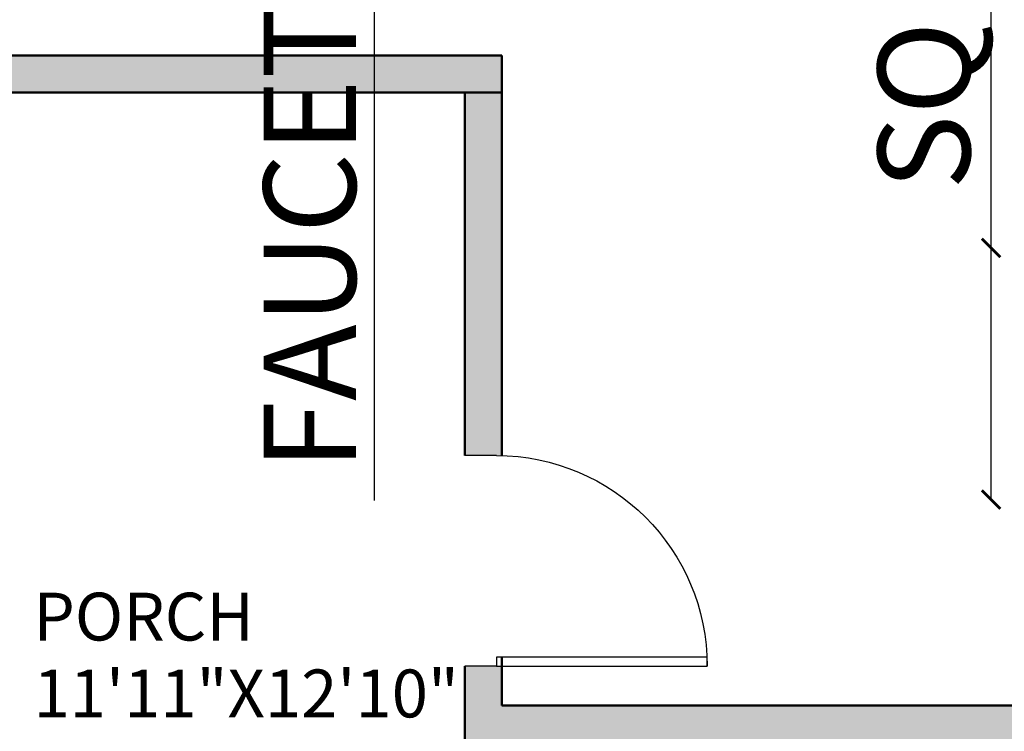
# Model space of a CAD drawing. Units: inches. Extents: x 2419 to 2878, y 1068 to 1713.
# Tile 9 of 20: x 2574 to 2708, y 1207 to 1304. Entities that reach past the tile are written whole.
import ezdxf

# ---------------------------------------------------------------- set-up
doc = ezdxf.new("R2010")
doc.units = ezdxf.units.IN
for name, color, linetype, lineweight in [('A-ANNO-DIMS', 2, 'Continuous', 18), ('A-AREA-IDEN', 7, 'Continuous', 18), ('A-DOOR', 4, 'Continuous', 25), ('A-FLOR-PRKG-PATT', 1, 'Continuous', 13), ('A-FURN-PATT', 254, 'Continuous', 13), ('A-WALL', 7, 'Continuous', 50)]:
    doc.layers.add(name, color=color, linetype=linetype, lineweight=lineweight)
doc.layers.add('A-FLOR-FIXT-PATT', color=254, linetype='Continuous', lineweight=13, true_color=0xd7ebd2)
doc.layers.add('A-WALL-PATT', color=18, linetype='Continuous', lineweight=13, true_color=0x000000)
doc.styles.get("Standard").update_dxf_attribs({"font": 'arial.ttf'})
doc.dimstyles.new('ISO-25', dxfattribs={"dimtxt": 12.5, "dimasz": 2.5, "dimexe": 1.25, "dimexo": 0.625, "dimtad": 1, "dimdec": 0, "dimlunit": 4, "dimtxsty": 'Standard', "dimblk": 'ARCHTICK', "dimcen": 2.5, "dimse1": 1, "dimse2": 1, "dimclrd": 4, "dimadec": 0, "dimazin": 0, "dimtfac": 1, "dimtdec": 0, "dimtmove": 0, "dimatfit": 3, "dimfxl": 1, "dimarcsym": 0})

# ---------------------------------------------------------------- blocks, each defined once
blk = doc.blocks.new('*U3')
for p, q in [((0, 0), (0, -6)), ((40, 0), (40, -6))]:
    blk.add_line(p, q)
blk.add_lwpolyline([(0, 0), (0, 40), (1.75, 40), (1.75, 0)], close=True)
blk.add_arc((0, 0), 40, 0, 90)
blk = doc.blocks.new('_ArchTick')
at = {"color": 0, "linetype": 'ByBlock', "const_width": 0.15}
blk.add_lwpolyline([(-0.5, -0.5), (0.5, 0.5)], dxfattribs=at)
blk = doc.blocks.new('*D20')
at = {"layer": 'A-ANNO-DIMS', "color": 4, "lineweight": -2, "transparency": 16777216}
for p, q in [((2622.22, 1404.52), (2622.22, 1392.52)), ((2622.22, 1392.52), (2622.22, 1238.58))]:
    blk.add_line(p, q, dxfattribs=at)
at = {"layer": 'Defpoints', "color": 0, "transparency": 16777216}
for p in [(2624.02, 1404.52), (2622.22, 1392.52), (2624.02, 1392.52)]:
    blk.add_point(p, dxfattribs=at)
at = {"layer": 'A-ANNO-DIMS', "color": 4, "lineweight": -2, "transparency": 16777216, "xscale": 2.5, "yscale": 2.5, "zscale": 2.5}
for p, rotation in [((2622.22, 1404.52), 90), ((2622.22, 1392.52), 270)]:
    blk.add_blockref('_ArchTick', p, dxfattribs=dict(at, rotation=rotation))
at = {"layer": 'A-ANNO-DIMS', "color": 0, "transparency": 16777216, "insert": (2615.13, 1314.3), "char_height": 12.5, "attachment_point": 5, "rotation": 90}
blk.add_mtext('FAUCET 1\'-0" TYP.', dxfattribs=at)
blk = doc.blocks.new('*D32')
at = {"layer": 'A-ANNO-DIMS', "color": 4, "lineweight": -2, "transparency": 16777216}
for p, q in [((2705.74, 1272.77), (2705.74, 1458.17)), ((2705.74, 1238.68), (2705.74, 1272.77))]:
    blk.add_line(p, q, dxfattribs=at)
at = {"layer": 'Defpoints', "color": 0, "transparency": 16777216}
for p in [(2705.74, 1272.77), (2710.85, 1272.77), (2710.85, 1238.68)]:
    blk.add_point(p, dxfattribs=at)
at = {"layer": 'A-ANNO-DIMS', "color": 4, "lineweight": -2, "transparency": 16777216, "xscale": 2.5, "yscale": 2.5, "zscale": 2.5}
for p, rotation in [((2705.74, 1272.77), 90), ((2705.74, 1238.68), 270)]:
    blk.add_blockref('_ArchTick', p, dxfattribs=dict(at, rotation=rotation))
at = {"layer": 'A-ANNO-DIMS', "color": 0, "transparency": 16777216, "insert": (2698.27, 1366.72), "char_height": 12.5, "attachment_point": 5, "rotation": 90}
blk.add_mtext('SQUARE TABLE 2\'-10"', dxfattribs=at)
blk = doc.blocks.new('*D36')
at = {"layer": 'A-ANNO-DIMS', "color": 4, "lineweight": -2, "transparency": 16777216}
blk.add_line((2656.74, 1605.01), (2736.32, 1605.01), dxfattribs=at)
at = {"layer": 'Defpoints', "color": 0, "transparency": 16777216}
for p in [(2736.32, 1605.01), (2656.74, 1205.81), (2736.32, 1205.81)]:
    blk.add_point(p, dxfattribs=at)
at = {"layer": 'A-ANNO-DIMS', "color": 4, "lineweight": -2, "transparency": 16777216, "xscale": 2.5, "yscale": 2.5, "zscale": 2.5, "rotation": 180}
blk.add_blockref('_ArchTick', (2656.74, 1605.01), dxfattribs=at)
at = {"layer": 'A-ANNO-DIMS', "color": 4, "lineweight": -2, "transparency": 16777216, "xscale": 2.5, "yscale": 2.5, "zscale": 2.5}
blk.add_blockref('_ArchTick', (2736.32, 1605.01), dxfattribs=at)
at = {"layer": 'A-ANNO-DIMS', "color": 0, "transparency": 16777216, "insert": (2696.53, 1612.1), "char_height": 12.5, "attachment_point": 5}
blk.add_mtext('6\'-7 1/2"', dxfattribs=at)
blk = doc.blocks.new('*D38')
at = {"layer": 'A-ANNO-DIMS', "color": 4, "lineweight": -2, "transparency": 16777216}
for p, q in [((2444.31, 1165.6), (2444.31, 1212.51)), ((2444.31, 1130.81), (2444.31, 1165.6))]:
    blk.add_line(p, q, dxfattribs=at)
at = {"layer": 'Defpoints', "color": 0, "transparency": 16777216}
for p in [(2444.31, 1165.6), (2656.74, 1165.6), (2656.74, 1130.81)]:
    blk.add_point(p, dxfattribs=at)
at = {"layer": 'A-ANNO-DIMS', "color": 4, "lineweight": -2, "transparency": 16777216, "xscale": 2.5, "yscale": 2.5, "zscale": 2.5}
for p, rotation in [((2444.31, 1165.6), 90), ((2444.31, 1130.81), 270)]:
    blk.add_blockref('_ArchTick', p, dxfattribs=dict(at, rotation=rotation))
at = {"layer": 'A-ANNO-DIMS', "color": 0, "transparency": 16777216, "insert": (2437.41, 1190.3), "char_height": 12.5, "attachment_point": 5, "rotation": 90}
blk.add_mtext('2\'-11"', dxfattribs=at)
blk = doc.blocks.new('*D39')
at = {"layer": 'A-ANNO-DIMS', "color": 4, "lineweight": -2, "transparency": 16777216}
for p, q in [((2662.74, 1605.01), (2668.59, 1605.01)), ((2668.59, 1605.01), (2705.56, 1605.01))]:
    blk.add_line(p, q, dxfattribs=at)
at = {"layer": 'Defpoints', "color": 0, "transparency": 16777216}
for p in [(2668.59, 1605.01), (2662.74, 1165.6), (2668.59, 1165.6)]:
    blk.add_point(p, dxfattribs=at)
at = {"layer": 'A-ANNO-DIMS', "color": 4, "lineweight": -2, "transparency": 16777216, "xscale": 2.5, "yscale": 2.5, "zscale": 2.5, "rotation": 180}
blk.add_blockref('_ArchTick', (2662.74, 1605.01), dxfattribs=at)
at = {"layer": 'A-ANNO-DIMS', "color": 4, "lineweight": -2, "transparency": 16777216, "xscale": 2.5, "yscale": 2.5, "zscale": 2.5}
blk.add_blockref('_ArchTick', (2668.59, 1605.01), dxfattribs=at)
at = {"layer": 'A-ANNO-DIMS', "color": 0, "transparency": 16777216, "insert": (2688.32, 1612.02), "char_height": 12.5, "attachment_point": 5}
blk.add_mtext('0\'-6"', dxfattribs=at)
blk = doc.blocks.new('*D44')
at = {"layer": 'A-ANNO-DIMS', "color": 4, "lineweight": -2, "transparency": 16777216}
for p, q in [((2557.3, 1079.92), (2585.82, 1079.92)), ((2585.82, 1079.92), (2652.14, 1079.92))]:
    blk.add_line(p, q, dxfattribs=at)
at = {"layer": 'Defpoints', "color": 0, "transparency": 16777216}
for p in [(2557.3, 1408.81), (2585.82, 1408.81), (2585.82, 1079.92)]:
    blk.add_point(p, dxfattribs=at)
at = {"layer": 'A-ANNO-DIMS', "color": 4, "lineweight": -2, "transparency": 16777216, "xscale": 2.5, "yscale": 2.5, "zscale": 2.5, "rotation": 180}
blk.add_blockref('_ArchTick', (2557.3, 1079.92), dxfattribs=at)
at = {"layer": 'A-ANNO-DIMS', "color": 4, "lineweight": -2, "transparency": 16777216, "xscale": 2.5, "yscale": 2.5, "zscale": 2.5}
blk.add_blockref('_ArchTick', (2585.82, 1079.92), dxfattribs=at)
at = {"layer": 'A-ANNO-DIMS', "color": 0, "transparency": 16777216, "insert": (2620.23, 1087.01), "char_height": 12.5, "attachment_point": 5}
blk.add_mtext('2\'-4 1/2"', dxfattribs=at)
blk = doc.blocks.new('*D45')
at = {"layer": 'A-ANNO-DIMS', "color": 4, "lineweight": -2, "transparency": 16777216}
for p, q in [((2596.57, 1079.92), (2625.09, 1079.92)), ((2625.09, 1079.92), (2691.41, 1079.92))]:
    blk.add_line(p, q, dxfattribs=at)
at = {"layer": 'Defpoints', "color": 0, "transparency": 16777216}
for p in [(2596.57, 1408.81), (2625.09, 1408.81), (2625.09, 1079.92)]:
    blk.add_point(p, dxfattribs=at)
at = {"layer": 'A-ANNO-DIMS', "color": 4, "lineweight": -2, "transparency": 16777216, "xscale": 2.5, "yscale": 2.5, "zscale": 2.5, "rotation": 180}
blk.add_blockref('_ArchTick', (2596.57, 1079.92), dxfattribs=at)
at = {"layer": 'A-ANNO-DIMS', "color": 4, "lineweight": -2, "transparency": 16777216, "xscale": 2.5, "yscale": 2.5, "zscale": 2.5}
blk.add_blockref('_ArchTick', (2625.09, 1079.92), dxfattribs=at)
at = {"layer": 'A-ANNO-DIMS', "color": 0, "transparency": 16777216, "insert": (2659.5, 1087.01), "char_height": 12.5, "attachment_point": 5}
blk.add_mtext('2\'-4 1/2"', dxfattribs=at)
blk = doc.blocks.new('*D47')
at = {"layer": 'A-ANNO-DIMS', "color": 4, "lineweight": -2, "transparency": 16777216}
for p, q in [((2444.31, 1376.56), (2444.31, 1357.98)), ((2444.31, 1357.98), (2444.31, 1293.05))]:
    blk.add_line(p, q, dxfattribs=at)
at = {"layer": 'Defpoints', "color": 0, "transparency": 16777216}
for p in [(2632.51, 1376.56), (2444.31, 1357.98), (2632.51, 1357.98)]:
    blk.add_point(p, dxfattribs=at)
at = {"layer": 'A-ANNO-DIMS', "color": 4, "lineweight": -2, "transparency": 16777216, "xscale": 2.5, "yscale": 2.5, "zscale": 2.5}
for p, rotation in [((2444.31, 1376.56), 90), ((2444.31, 1357.98), 270)]:
    blk.add_blockref('_ArchTick', p, dxfattribs=dict(at, rotation=rotation))
at = {"layer": 'A-ANNO-DIMS', "color": 0, "transparency": 16777216, "insert": (2437.23, 1324.26), "char_height": 12.5, "attachment_point": 5, "rotation": 90}
blk.add_mtext('1\'-6 1/2"', dxfattribs=at)
blk = doc.blocks.new('*D53')
at = {"layer": 'A-ANNO-DIMS', "color": 4, "lineweight": -2, "transparency": 16777216}
for p, q in [((2638.79, 1605.01), (2667.31, 1605.01)), ((2667.31, 1605.01), (2733.63, 1605.01))]:
    blk.add_line(p, q, dxfattribs=at)
at = {"layer": 'Defpoints', "color": 0, "transparency": 16777216}
for p in [(2667.31, 1605.01), (2638.79, 1217.38), (2667.31, 1217.38)]:
    blk.add_point(p, dxfattribs=at)
at = {"layer": 'A-ANNO-DIMS', "color": 4, "lineweight": -2, "transparency": 16777216, "xscale": 2.5, "yscale": 2.5, "zscale": 2.5, "rotation": 180}
blk.add_blockref('_ArchTick', (2638.79, 1605.01), dxfattribs=at)
at = {"layer": 'A-ANNO-DIMS', "color": 4, "lineweight": -2, "transparency": 16777216, "xscale": 2.5, "yscale": 2.5, "zscale": 2.5}
blk.add_blockref('_ArchTick', (2667.31, 1605.01), dxfattribs=at)
at = {"layer": 'A-ANNO-DIMS', "color": 0, "transparency": 16777216, "insert": (2701.72, 1612.1), "char_height": 12.5, "attachment_point": 5}
blk.add_mtext('2\'-4 1/2"', dxfattribs=at)
blk = doc.blocks.new('*D56')
at = {"layer": 'A-ANNO-DIMS', "color": 4, "lineweight": -2, "transparency": 16777216}
for p, q in [((2480.51, 1079.92), (2503.97, 1079.92)), ((2503.97, 1079.92), (2578.61, 1079.92))]:
    blk.add_line(p, q, dxfattribs=at)
at = {"layer": 'Defpoints', "color": 0, "transparency": 16777216}
for p in [(2480.51, 1507.81), (2503.97, 1494.85), (2503.97, 1079.92)]:
    blk.add_point(p, dxfattribs=at)
at = {"layer": 'A-ANNO-DIMS', "color": 4, "lineweight": -2, "transparency": 16777216, "xscale": 2.5, "yscale": 2.5, "zscale": 2.5, "rotation": 180}
blk.add_blockref('_ArchTick', (2480.51, 1079.92), dxfattribs=at)
at = {"layer": 'A-ANNO-DIMS', "color": 4, "lineweight": -2, "transparency": 16777216, "xscale": 2.5, "yscale": 2.5, "zscale": 2.5}
blk.add_blockref('_ArchTick', (2503.97, 1079.92), dxfattribs=at)
at = {"layer": 'A-ANNO-DIMS', "color": 0, "transparency": 16777216, "insert": (2542.54, 1087.01), "char_height": 12.5, "attachment_point": 5}
blk.add_mtext('1\'-11 1/2"', dxfattribs=at)
blk = doc.blocks.new('*D59')
at = {"layer": 'A-ANNO-DIMS', "color": 4, "lineweight": -2, "transparency": 16777216}
blk.add_line((2480.51, 1079.92), (2589.51, 1079.92), dxfattribs=at)
at = {"layer": 'Defpoints', "color": 0, "transparency": 16777216}
for p in [(2480.51, 1414.81), (2589.51, 1414.81), (2589.51, 1079.92)]:
    blk.add_point(p, dxfattribs=at)
at = {"layer": 'A-ANNO-DIMS', "color": 4, "lineweight": -2, "transparency": 16777216, "xscale": 2.5, "yscale": 2.5, "zscale": 2.5, "rotation": 180}
blk.add_blockref('_ArchTick', (2480.51, 1079.92), dxfattribs=at)
at = {"layer": 'A-ANNO-DIMS', "color": 4, "lineweight": -2, "transparency": 16777216, "xscale": 2.5, "yscale": 2.5, "zscale": 2.5}
blk.add_blockref('_ArchTick', (2589.51, 1079.92), dxfattribs=at)
at = {"layer": 'A-ANNO-DIMS', "color": 0, "transparency": 16777216, "insert": (2535.01, 1086.93), "char_height": 12.5, "attachment_point": 5}
blk.add_mtext('9\'-1"', dxfattribs=at)

msp = doc.modelspace()

# ---------------------------------------------------------------- hatches: boundary and pattern name
at = {"layer": 'A-FLOR-FIXT-PATT'}
h = msp.add_hatch(color=256, dxfattribs=at)
h.dxf.hatch_style = 1
h.paths.add_polyline_path([(2771.51, 1458.39), (2763.51, 1458.39), (2763.51, 1437.39), (2771.51, 1437.39)])
h.paths.add_polyline_path([(2770.51, 1456.39, 0.5), (2769.51, 1457.39), (2765.51, 1457.39, 0.5), (2764.51, 1456.39), (2764.51, 1439.39, 0.5), (2765.51, 1438.39), (2769.51, 1438.39, 0.5), (2770.51, 1439.39)], flags=16)
h.paths.add_polyline_path([(2706.38, 1408.81), (2685.38, 1408.81), (2685.38, 1400.81), (2706.38, 1400.81)])
h.paths.add_polyline_path([(2704.38, 1401.81, 0.5), (2705.38, 1402.81), (2705.38, 1406.81, 0.5), (2704.38, 1407.81), (2687.38, 1407.81, 0.5), (2686.38, 1406.81), (2686.38, 1402.81, 0.5), (2687.38, 1401.81)], flags=16)
h.paths.add_polyline_path([(2574.48, 1207.45), (2633.94, 1207.45), (2633.94, 1217.37), (2574.48, 1217.37)], flags=9)
h.paths.add_polyline_path([(2574.45, 1217.83), (2610.47, 1217.83), (2610.47, 1227.88), (2574.45, 1227.88)], flags=9)
h.paths.add_polyline_path([(2672.43, 1304.02), (2718.62, 1304.02), (2718.62, 1313.94), (2672.43, 1313.94)], flags=9)
h.paths.add_polyline_path([(2672.4, 1314.4), (2750.13, 1314.4), (2750.13, 1324.45), (2672.4, 1324.45)], flags=9)
h.paths.add_polyline_path([(2500.43, 1374.44), (2544.8, 1374.44), (2544.8, 1384.36), (2500.43, 1384.36)], flags=9)
h.paths.add_polyline_path([(2500.41, 1384.82), (2566.08, 1384.82), (2566.08, 1394.87), (2500.41, 1394.87)], flags=9)
h.paths.add_polyline_path([(2738.93, 1376.75), (2778.27, 1376.75), (2778.27, 1386.67), (2738.93, 1386.67)], flags=9)
h.paths.add_polyline_path([(2659.12, 1357.8), (2703.49, 1357.8), (2703.49, 1367.72), (2659.12, 1367.72)], flags=9)
h.paths.add_polyline_path([(2659.1, 1368.18), (2694.11, 1368.18), (2694.11, 1378.23), (2659.1, 1378.23)], flags=9)
h.paths.add_polyline_path([(2730.12, 1466.07), (2769.46, 1466.07), (2769.46, 1475.99), (2730.12, 1475.99)], flags=9)
h.paths.add_polyline_path([(2730.1, 1476.45), (2765.12, 1476.45), (2765.12, 1486.5), (2730.1, 1486.5)], flags=9)
h.paths.add_polyline_path([(2730.38, 1518.65), (2761.48, 1518.65), (2761.48, 1528.57), (2730.38, 1528.57)], flags=9)
h.paths.add_polyline_path([(2730.36, 1529.03), (2780.96, 1529.03), (2780.96, 1539.07), (2730.36, 1539.07)], flags=9)
h.paths.add_polyline_path([(2629.32, 1455.19), (2688.78, 1455.19), (2688.78, 1465.11), (2629.32, 1465.11)], flags=9)
h.paths.add_polyline_path([(2629.3, 1465.57), (2681.9, 1465.57), (2681.9, 1475.62), (2629.3, 1475.62)], flags=9)
h.paths.add_polyline_path([(2513.23, 1456.48), (2562.63, 1456.48), (2562.63, 1466.4), (2513.23, 1466.4)], flags=9)
h.paths.add_polyline_path([(2513.21, 1466.86), (2556.26, 1466.86), (2556.26, 1476.91), (2513.21, 1476.91)], flags=9)
h.paths.add_polyline_path([(2488.87, 1521.54), (2519.97, 1521.54), (2519.97, 1531.46), (2488.87, 1531.46)], flags=9)
h.paths.add_polyline_path([(2536.55, 1543.51), (2580.92, 1543.51), (2580.92, 1553.43), (2536.55, 1553.43)], flags=9)
h.paths.add_polyline_path([(2536.56, 1553.92), (2573.53, 1553.92), (2573.53, 1563.8), (2536.56, 1563.8)], flags=9)
at = {"layer": 'A-FLOR-PRKG-PATT'}
h = msp.add_hatch(color=256, dxfattribs=at)
h.dxf.hatch_style = 1
edge = h.paths.add_edge_path()
edge.add_ellipse((2561.37, 1279.45), major_axis=(3.99, 0), ratio=0.842304, start_angle=0.6466, end_angle=90)
edge.add_line((2561.37, 1282.81), (2511.57, 1282.81))
edge.add_ellipse((2511.57, 1279.45), major_axis=(3.99, 0), ratio=0.842304, start_angle=90, end_angle=179.3534)
edge.add_ellipse((10560.89, 1188.62), major_axis=(-8054.03, 0), ratio=0.8423039, start_angle=-0.646554, end_angle=-0.628237)
edge.add_ellipse((2509.23, 1276.91), major_axis=(1.69, 0), ratio=0.842304, start_angle=179.3718, end_angle=248.4648)
edge.add_ellipse((10560.33, 1188.62), major_axis=(8052.29, 0), ratio=0.8423039, start_angle=179.353446, end_angle=179.381357, ccw=False)
edge.add_ellipse((2511.01, 1279.45), major_axis=(2.25, 0), ratio=0.842304, start_angle=90, end_angle=179.3534, ccw=False)
edge.add_line((2511.01, 1281.35), (2561.94, 1281.35))
edge.add_ellipse((2561.94, 1279.45), major_axis=(-2.25, 0), ratio=0.842304, start_angle=180.6466, end_angle=270, ccw=False)
edge.add_ellipse((-5487.38, 1188.62), major_axis=(8052.29, 0), ratio=0.8423039, start_angle=0.528271, end_angle=0.646554, ccw=False)
edge.add_ellipse((2563.71, 1276.91), major_axis=(-1.69, 0), ratio=0.842304, start_angle=111.5352, end_angle=180.6282)
edge.add_ellipse((-5487.95, 1188.62), major_axis=(-8054.03, 0), ratio=0.8423039, start_angle=180.628237, end_angle=180.646554)
edge = h.paths.add_edge_path()
edge.add_ellipse((2564.91, 1261.91), major_axis=(-1.12, 0), ratio=0.842304, start_angle=180, end_angle=270)
edge.add_line((2564.91, 1262.86), (2564.43, 1262.86))
edge.add_ellipse((-5487.38, 1188.62), major_axis=(8052.29, 0), ratio=0.8423039, start_angle=0.383867, end_angle=0.528271, ccw=False)
edge.add_line((2564.65, 1242.56), (2564.91, 1242.56))
edge.add_ellipse((2564.91, 1243.51), major_axis=(-1.12, 0), ratio=0.842304, start_angle=90, end_angle=180)
edge.add_line((2566.03, 1243.51), (2566.03, 1261.91))
edge = h.paths.add_edge_path()
edge.add_ellipse((2564.91, 1174.99), major_axis=(1.12, 0), ratio=0.842304, start_angle=0, end_angle=90)
edge.add_line((2564.91, 1175.94), (2564.89, 1175.94))
edge.add_ellipse((-5487.38, 1188.62), major_axis=(8052.29, 0), ratio=0.8423039, start_angle=-0.134987, end_angle=-0.090229, ccw=False)
edge.add_ellipse((2163.34, 1170.91), major_axis=(401.54, 0), ratio=0.842304, start_angle=-2.18, end_angle=-0.1356, ccw=False)
edge.add_line((2564.47, 1155.64), (2564.91, 1155.64))
edge.add_ellipse((2564.91, 1156.59), major_axis=(-1.12, 0), ratio=0.842304, start_angle=90, end_angle=180)
edge.add_line((2566.03, 1156.59), (2566.03, 1174.99))
h.paths.add_polyline_path([(2574.48, 1207.45), (2633.94, 1207.45), (2633.94, 1217.37), (2574.48, 1217.37)], flags=9)
h.paths.add_polyline_path([(2574.45, 1217.83), (2610.47, 1217.83), (2610.47, 1227.88), (2574.45, 1227.88)], flags=9)
h.paths.add_polyline_path([(2672.43, 1304.02), (2718.62, 1304.02), (2718.62, 1313.94), (2672.43, 1313.94)], flags=9)
h.paths.add_polyline_path([(2672.4, 1314.4), (2750.13, 1314.4), (2750.13, 1324.45), (2672.4, 1324.45)], flags=9)
h.paths.add_polyline_path([(2500.43, 1374.44), (2544.8, 1374.44), (2544.8, 1384.36), (2500.43, 1384.36)], flags=9)
h.paths.add_polyline_path([(2500.41, 1384.82), (2566.08, 1384.82), (2566.08, 1394.87), (2500.41, 1394.87)], flags=9)
h.paths.add_polyline_path([(2738.93, 1376.75), (2778.27, 1376.75), (2778.27, 1386.67), (2738.93, 1386.67)], flags=9)
h.paths.add_polyline_path([(2659.12, 1357.8), (2703.49, 1357.8), (2703.49, 1367.72), (2659.12, 1367.72)], flags=9)
h.paths.add_polyline_path([(2659.1, 1368.18), (2694.11, 1368.18), (2694.11, 1378.23), (2659.1, 1378.23)], flags=9)
h.paths.add_polyline_path([(2730.12, 1466.07), (2769.46, 1466.07), (2769.46, 1475.99), (2730.12, 1475.99)], flags=9)
h.paths.add_polyline_path([(2730.1, 1476.45), (2765.12, 1476.45), (2765.12, 1486.5), (2730.1, 1486.5)], flags=9)
h.paths.add_polyline_path([(2730.38, 1518.65), (2761.48, 1518.65), (2761.48, 1528.57), (2730.38, 1528.57)], flags=9)
h.paths.add_polyline_path([(2730.36, 1529.03), (2780.96, 1529.03), (2780.96, 1539.07), (2730.36, 1539.07)], flags=9)
h.paths.add_polyline_path([(2629.32, 1455.19), (2688.78, 1455.19), (2688.78, 1465.11), (2629.32, 1465.11)], flags=9)
h.paths.add_polyline_path([(2629.3, 1465.57), (2681.9, 1465.57), (2681.9, 1475.62), (2629.3, 1475.62)], flags=9)
h.paths.add_polyline_path([(2513.23, 1456.48), (2562.63, 1456.48), (2562.63, 1466.4), (2513.23, 1466.4)], flags=9)
h.paths.add_polyline_path([(2513.21, 1466.86), (2556.26, 1466.86), (2556.26, 1476.91), (2513.21, 1476.91)], flags=9)
h.paths.add_polyline_path([(2488.87, 1521.54), (2519.97, 1521.54), (2519.97, 1531.46), (2488.87, 1531.46)], flags=9)
h.paths.add_polyline_path([(2536.55, 1543.51), (2580.92, 1543.51), (2580.92, 1553.43), (2536.55, 1553.43)], flags=9)
h.paths.add_polyline_path([(2536.56, 1553.92), (2573.53, 1553.92), (2573.53, 1563.8), (2536.56, 1563.8)], flags=9)
at = {"layer": 'A-FURN-PATT'}
h = msp.add_hatch(color=256, dxfattribs=at)
h.dxf.hatch_style = 1
h.paths.add_polyline_path([(2710.17, 1562.64), (2707.17, 1559.64), (2709.17, 1559.64, -0.414214), (2710.17, 1560.64)])
h.paths.add_polyline_path([(2711.17, 1559.64, 1), (2709.17, 1559.64, 1)])
h.paths.add_polyline_path([(2710.17, 1562.64), (2710.17, 1560.64, -0.414214), (2711.17, 1559.64), (2713.17, 1559.64)])
h.paths.add_polyline_path([(2713.17, 1559.64), (2711.17, 1559.64, -0.414214), (2710.17, 1558.64), (2710.17, 1556.64)])
h.paths.add_polyline_path([(2710.17, 1558.64, -0.414214), (2709.17, 1559.64), (2707.17, 1559.64), (2710.17, 1556.64)])
h.paths.add_polyline_path([(2613.13, 1558.89, 1), (2611.13, 1558.89, 1)])
h.paths.add_polyline_path([(2612.13, 1561.89), (2612.13, 1559.89, -0.414214), (2613.13, 1558.89), (2615.13, 1558.89)])
h.paths.add_polyline_path([(2612.13, 1559.89), (2612.13, 1561.89), (2609.13, 1558.89), (2611.13, 1558.89, -0.414214)])
h.paths.add_polyline_path([(2612.13, 1557.89, -0.414214), (2611.13, 1558.89), (2609.13, 1558.89), (2612.13, 1555.89)])
h.paths.add_polyline_path([(2574.48, 1207.45), (2633.94, 1207.45), (2633.94, 1217.37), (2574.48, 1217.37)], flags=9)
h.paths.add_polyline_path([(2574.45, 1217.83), (2610.47, 1217.83), (2610.47, 1227.88), (2574.45, 1227.88)], flags=9)
h.paths.add_polyline_path([(2672.43, 1304.02), (2718.62, 1304.02), (2718.62, 1313.94), (2672.43, 1313.94)], flags=9)
h.paths.add_polyline_path([(2672.4, 1314.4), (2750.13, 1314.4), (2750.13, 1324.45), (2672.4, 1324.45)], flags=9)
h.paths.add_polyline_path([(2500.43, 1374.44), (2544.8, 1374.44), (2544.8, 1384.36), (2500.43, 1384.36)], flags=9)
h.paths.add_polyline_path([(2500.41, 1384.82), (2566.08, 1384.82), (2566.08, 1394.87), (2500.41, 1394.87)], flags=9)
h.paths.add_polyline_path([(2738.93, 1376.75), (2778.27, 1376.75), (2778.27, 1386.67), (2738.93, 1386.67)], flags=9)
h.paths.add_polyline_path([(2659.12, 1357.8), (2703.49, 1357.8), (2703.49, 1367.72), (2659.12, 1367.72)], flags=9)
h.paths.add_polyline_path([(2659.1, 1368.18), (2694.11, 1368.18), (2694.11, 1378.23), (2659.1, 1378.23)], flags=9)
h.paths.add_polyline_path([(2730.12, 1466.07), (2769.46, 1466.07), (2769.46, 1475.99), (2730.12, 1475.99)], flags=9)
h.paths.add_polyline_path([(2730.1, 1476.45), (2765.12, 1476.45), (2765.12, 1486.5), (2730.1, 1486.5)], flags=9)
h.paths.add_polyline_path([(2730.38, 1518.65), (2761.48, 1518.65), (2761.48, 1528.57), (2730.38, 1528.57)], flags=9)
h.paths.add_polyline_path([(2730.36, 1529.03), (2780.96, 1529.03), (2780.96, 1539.07), (2730.36, 1539.07)], flags=9)
h.paths.add_polyline_path([(2629.32, 1455.19), (2688.78, 1455.19), (2688.78, 1465.11), (2629.32, 1465.11)], flags=9)
h.paths.add_polyline_path([(2629.3, 1465.57), (2681.9, 1465.57), (2681.9, 1475.62), (2629.3, 1475.62)], flags=9)
h.paths.add_polyline_path([(2513.23, 1456.48), (2562.63, 1456.48), (2562.63, 1466.4), (2513.23, 1466.4)], flags=9)
h.paths.add_polyline_path([(2513.21, 1466.86), (2556.26, 1466.86), (2556.26, 1476.91), (2513.21, 1476.91)], flags=9)
h.paths.add_polyline_path([(2488.87, 1521.54), (2519.97, 1521.54), (2519.97, 1531.46), (2488.87, 1531.46)], flags=9)
h.paths.add_polyline_path([(2536.55, 1543.51), (2580.92, 1543.51), (2580.92, 1553.43), (2536.55, 1553.43)], flags=9)
h.paths.add_polyline_path([(2536.56, 1553.92), (2573.53, 1553.92), (2573.53, 1563.8), (2536.56, 1563.8)], flags=9)
at = {"layer": 'A-WALL-PATT'}
h = msp.add_hatch(color=256, dxfattribs=at)
h.dxf.hatch_style = 1
h.paths.add_polyline_path([(2780.51, 1577.81), (2471.51, 1577.81), (2471.51, 1121.81), (2780.51, 1121.81)])
h.paths.add_polyline_path([(2480.51, 1568.81), (2771.51, 1568.81), (2771.51, 1130.81), (2480.51, 1130.81)], flags=16)
h.paths.add_polyline_path([(2528.51, 1568.81), (2528.51, 1512.81), (2594.51, 1512.81), (2594.51, 1414.81), (2596.57, 1414.81), (2596.57, 1441.61), (2597.82, 1441.61), (2597.82, 1441.58, -0.384016), (2625.03, 1414.81), (2725.51, 1414.81), (2725.51, 1567.55), (2728.3, 1567.55), (2746.89, 1567.55), (2746.89, 1566.73), (2746.87, 1566.73, -0.367216), (2730.51, 1549.09), (2730.51, 1512.81), (2750.85, 1512.81), (2750.85, 1510.03, -0.401453), (2733.08, 1491.46), (2733.08, 1491.44), (2732.27, 1491.44), (2732.27, 1507.81), (2730.51, 1507.81), (2730.51, 1408.81), (2736.51, 1408.81), (2736.51, 1349.81), (2632.51, 1349.81), (2632.51, 1408.81), (2528.51, 1408.81), (2528.51, 1414.81), (2503.97, 1414.81), (2503.97, 1494.85), (2558.38, 1494.85), (2558.38, 1507.81), (2529.96, 1507.81, -0.414214), (2530.82, 1506.96), (2530.82, 1497.26, -0.414214), (2529.96, 1496.4), (2514.56, 1496.4, -0.414214), (2513.7, 1497.26), (2513.7, 1506.96, -0.414214), (2514.56, 1507.81), (2528.51, 1507.81), (2528.51, 1512.81), (2480.51, 1512.81)], flags=0)
h.paths.add_polyline_path([(2516.26, 1507.81), (2528.26, 1507.81), (2528.26, 1505.81), (2523.42, 1505.81), (2524.07, 1504.67), (2529.39, 1504.67, -0.414214), (2529.96, 1504.1), (2529.96, 1497.83, -0.414214), (2529.39, 1497.26), (2515.13, 1497.26, -0.414214), (2514.56, 1497.83), (2514.56, 1504.1, -0.414214), (2515.13, 1504.67), (2520.69, 1504.67), (2521.34, 1505.81), (2516.26, 1505.81)], flags=0)
h.paths.add_polyline_path([(2522.02, 1505.53), (2522.82, 1507.32, -0.65506), (2522.25, 1506.06), (2522.19, 1505.93), (2522.43, 1505.53)], flags=0)
h.paths.add_polyline_path([(2522.83, 1500.97, -1), (2521.69, 1500.97, -1)], flags=0)
h.paths.add_polyline_path([(2522.55, 1500.97, -1), (2521.98, 1500.97, -1)], flags=0)
h.paths.add_polyline_path([(2482.01, 1470.63), (2499.89, 1470.63), (2499.89, 1448.27), (2482.01, 1448.27), (2482.01, 1452.74), (2481.26, 1452.74), (2481.26, 1449.76), (2480.51, 1449.76), (2480.51, 1469.14), (2481.26, 1469.14), (2481.26, 1466.16), (2482.01, 1466.16)], flags=0)
h.paths.add_polyline_path([(2488.71, 1466.16, -1), (2484.24, 1466.16, -1)], flags=0)
h.paths.add_polyline_path([(2496.17, 1466.16, -1), (2490.2, 1466.16, -1)], flags=0)
h.paths.add_polyline_path([(2487.97, 1466.16, -1), (2484.99, 1466.16, -1)], flags=0)
h.paths.add_polyline_path([(2495.42, 1466.16, -1), (2490.95, 1466.16, -1)], flags=0)
h.paths.add_polyline_path([(2487.22, 1466.16, -1), (2485.73, 1466.16, -1)], flags=0)
h.paths.add_polyline_path([(2494.68, 1466.16, -1), (2491.69, 1466.16, -1)], flags=0)
h.paths.add_polyline_path([(2499.11, 1468, -1), (2497.98, 1468, -1)], flags=0)
h.paths.add_polyline_path([(2493.93, 1466.16, -1), (2492.44, 1466.16, -1)], flags=0)
h.paths.add_polyline_path([(2499.37, 1463.71, -1), (2498.17, 1463.71, -1)], flags=0)
h.paths.add_polyline_path([(2484.24, 1461.69), (2496.17, 1461.69), (2496.17, 1457.22), (2484.24, 1457.22)], flags=0)
h.paths.add_polyline_path([(2484.99, 1460.94), (2495.42, 1460.94), (2495.42, 1457.96), (2484.99, 1457.96)], flags=0)
h.paths.add_polyline_path([(2586.88, 1510.03), (2587.69, 1510.03), (2587.69, 1491.44), (2586.88, 1491.44)], flags=0)
h.paths.add_polyline_path([(2499.26, 1459.41, -1), (2498.2, 1459.41, -1)], flags=0)
h.paths.add_polyline_path([(2489.46, 1452.74, -1), (2483.5, 1452.74, -1)], flags=0)
h.paths.add_polyline_path([(2557.3, 1408.81), (2557.3, 1413.09, -0.401453), (2584.57, 1441.58), (2584.57, 1441.61), (2585.82, 1441.61), (2585.82, 1413.09), (2585.82, 1408.81)], flags=0)
h.paths.add_polyline_path([(2488.71, 1452.74, -1), (2484.24, 1452.74, -1)], flags=0)
h.paths.add_polyline_path([(2495.42, 1452.74, -1), (2490.95, 1452.74, -1)], flags=0)
h.paths.add_polyline_path([(2487.97, 1452.74, -1), (2484.99, 1452.74, -1)], flags=0)
h.paths.add_polyline_path([(2494.68, 1452.74, -1), (2491.69, 1452.74, -1)], flags=0)
h.paths.add_polyline_path([(2487.22, 1452.74, -1), (2485.73, 1452.74, -1)], flags=0)
h.paths.add_polyline_path([(2499.18, 1454.44, -1), (2497.9, 1454.44, -1)], flags=0)
h.paths.add_polyline_path([(2493.93, 1452.74, -1), (2492.44, 1452.74, -1)], flags=0)
h.paths.add_polyline_path([(2499.3, 1450.64, -1), (2497.79, 1450.64, -1)], flags=0)
h.paths.add_polyline_path([(2619.13, 1558.89, -1), (2605.13, 1558.89, -1)], flags=0)
h.paths.add_polyline_path([(2609.13, 1558.89), (2612.13, 1561.89), (2615.13, 1558.89), (2612.13, 1555.89)], flags=0)
h.paths.add_polyline_path([(2611.13, 1558.89, -1), (2613.13, 1558.89, -1)], flags=0)
h.paths.add_polyline_path([(2633.68, 1568.81), (2693.68, 1568.81), (2693.68, 1488.81), (2633.68, 1488.81)], flags=0)
h.paths.add_polyline_path([(2641.68, 1554.41), (2641.68, 1567.61), (2662.48, 1567.61), (2662.48, 1554.41), (2664.88, 1554.41), (2664.88, 1567.61), (2685.68, 1567.61), (2685.68, 1552.41), (2680.48, 1552.41), (2693.68, 1539.21), (2678.48, 1539.21), (2678.48, 1554.41)], flags=0)
h.paths.add_polyline_path([(2637.51, 1408.81), (2731.51, 1408.81), (2731.51, 1354.81), (2637.51, 1354.81), (2637.51, 1357.98), (2635.3, 1357.98), (2635.3, 1358.79), (2637.51, 1358.79)], flags=0)
h.paths.add_polyline_path([(2717.17, 1559.64, -1), (2703.17, 1559.64, -1)], flags=0)
h.paths.add_polyline_path([(2707.17, 1559.64), (2710.17, 1562.64), (2713.17, 1559.64), (2710.17, 1556.64)], flags=0)
h.paths.add_polyline_path([(2709.17, 1559.64, -1), (2711.17, 1559.64, -1)], flags=0)
h.paths.add_polyline_path([(2685.38, 1408.81), (2706.38, 1408.81), (2706.38, 1400.81), (2699.88, 1400.81), (2701.88, 1394.81, -0.501323), (2696.92, 1375.95, -0.132891), (2694.83, 1375.95, -0.501317), (2689.88, 1394.81), (2691.88, 1400.81), (2688.88, 1400.81), (2688.88, 1399.31), (2685.88, 1399.31), (2685.88, 1400.31), (2687.88, 1400.31), (2687.88, 1400.81), (2685.38, 1400.81)], flags=0)
h.paths.add_polyline_path([(2687.38, 1407.81), (2704.38, 1407.81, -0.5), (2705.38, 1406.81), (2705.38, 1402.81, -0.5), (2704.38, 1401.81), (2687.38, 1401.81, -0.5), (2686.38, 1402.81), (2686.38, 1406.81, -0.5)], flags=0)
h.paths.add_polyline_path([(2639.51, 1205.81), (2634.51, 1205.81), (2634.51, 1293.81), (2637.51, 1293.81), (2639.51, 1293.81)], flags=0)
h.paths.add_polyline_path([(2691.88, 1394.81), (2699.88, 1394.81, -0.48008), (2697.52, 1377.29, -0.215004), (2694.23, 1377.29, -0.48008)], flags=0)
h.paths.add_polyline_path([(2757.51, 1453.89), (2763.51, 1451.89), (2763.51, 1454.89), (2762.01, 1454.89), (2762.01, 1457.89), (2763.01, 1457.89), (2763.01, 1455.89), (2763.51, 1455.89), (2763.51, 1458.39), (2771.51, 1458.39), (2771.51, 1437.39), (2763.51, 1437.39), (2763.51, 1443.89), (2757.51, 1441.89, -0.501323), (2738.65, 1446.85, -0.132891), (2738.65, 1448.94, -0.501317)], flags=0)
h.paths.add_polyline_path([(2739.99, 1449.54, -0.48008), (2757.51, 1451.89), (2757.51, 1443.89, -0.48008), (2739.99, 1446.25, -0.215004)], flags=0)
h.paths.add_polyline_path([(2765.51, 1457.39), (2769.51, 1457.39, -0.5), (2770.51, 1456.39), (2770.51, 1439.39, -0.5), (2769.51, 1438.39), (2765.51, 1438.39, -0.5), (2764.51, 1439.39), (2764.51, 1456.39, -0.5)], flags=0)
h = msp.add_hatch(color=256, dxfattribs=at)
h.dxf.hatch_style = 1
h.paths.add_polyline_path([(2771.51, 1354.81), (2736.51, 1354.81), (2736.51, 1408.81), (2771.51, 1408.81), (2771.51, 1414.81), (2625.03, 1414.81, -0.015108), (2625.09, 1413.09), (2625.09, 1408.81), (2632.51, 1408.81), (2632.51, 1376.56), (2635.3, 1376.56, -0.029838), (2637.51, 1376.43), (2637.51, 1408.81), (2731.51, 1408.81), (2731.51, 1354.81), (2637.51, 1354.81), (2637.51, 1357.98), (2635.3, 1357.98), (2632.51, 1357.98), (2632.51, 1349.81), (2771.51, 1349.81)])
h.paths.add_polyline_path([(2639.51, 1298.81), (2637.51, 1298.81), (2480.51, 1298.81), (2480.51, 1293.81), (2637.51, 1293.81), (2639.51, 1293.81)])
h.paths.add_polyline_path([(2639.51, 1293.81), (2637.51, 1293.81), (2634.51, 1293.81), (2634.51, 1244.65), (2638.79, 1244.65, -0.006332), (2639.51, 1244.64)])
h.paths.add_polyline_path([(2639.51, 1205.81), (2771.51, 1205.81), (2771.51, 1210.81), (2639.51, 1210.81), (2639.51, 1216.13), (2638.79, 1216.13), (2634.51, 1216.13), (2634.51, 1130.81), (2639.51, 1130.81)])
h.paths.add_polyline_path([(2596.57, 1413.09), (2596.57, 1414.81), (2585.82, 1414.81), (2585.82, 1413.09), (2585.82, 1408.81), (2596.57, 1408.81)])
h.paths.add_polyline_path([(2557.3, 1413.09, -0.015108), (2557.35, 1414.81), (2480.51, 1414.81), (2480.51, 1408.81), (2557.3, 1408.81)])
h.paths.add_polyline_path([(2574.48, 1207.45), (2633.94, 1207.45), (2633.94, 1217.37), (2574.48, 1217.37)], flags=9)
h.paths.add_polyline_path([(2574.45, 1217.83), (2610.47, 1217.83), (2610.47, 1227.88), (2574.45, 1227.88)], flags=9)
h.paths.add_polyline_path([(2672.43, 1304.02), (2718.62, 1304.02), (2718.62, 1313.94), (2672.43, 1313.94)], flags=9)
h.paths.add_polyline_path([(2672.4, 1314.4), (2750.13, 1314.4), (2750.13, 1324.45), (2672.4, 1324.45)], flags=9)
h.paths.add_polyline_path([(2500.43, 1374.44), (2544.8, 1374.44), (2544.8, 1384.36), (2500.43, 1384.36)], flags=9)
h.paths.add_polyline_path([(2500.41, 1384.82), (2566.08, 1384.82), (2566.08, 1394.87), (2500.41, 1394.87)], flags=9)
h.paths.add_polyline_path([(2738.93, 1376.75), (2778.27, 1376.75), (2778.27, 1386.67), (2738.93, 1386.67)], flags=9)
h.paths.add_polyline_path([(2659.12, 1357.8), (2703.49, 1357.8), (2703.49, 1367.72), (2659.12, 1367.72)], flags=25)
h.paths.add_polyline_path([(2659.1, 1368.18), (2694.11, 1368.18), (2694.11, 1378.23), (2659.1, 1378.23)], flags=25)
h.paths.add_polyline_path([(2730.12, 1466.07), (2769.46, 1466.07), (2769.46, 1475.99), (2730.12, 1475.99)], flags=9)
h.paths.add_polyline_path([(2730.1, 1476.45), (2765.12, 1476.45), (2765.12, 1486.5), (2730.1, 1486.5)], flags=9)
h.paths.add_polyline_path([(2730.38, 1518.65), (2761.48, 1518.65), (2761.48, 1528.57), (2730.38, 1528.57)], flags=9)
h.paths.add_polyline_path([(2730.36, 1529.03), (2780.96, 1529.03), (2780.96, 1539.07), (2730.36, 1539.07)], flags=9)
h.paths.add_polyline_path([(2629.32, 1455.19), (2688.78, 1455.19), (2688.78, 1465.11), (2629.32, 1465.11)], flags=9)
h.paths.add_polyline_path([(2629.3, 1465.57), (2681.9, 1465.57), (2681.9, 1475.62), (2629.3, 1475.62)], flags=9)
h.paths.add_polyline_path([(2513.23, 1456.48), (2562.63, 1456.48), (2562.63, 1466.4), (2513.23, 1466.4)], flags=9)
h.paths.add_polyline_path([(2513.21, 1466.86), (2556.26, 1466.86), (2556.26, 1476.91), (2513.21, 1476.91)], flags=9)
h.paths.add_polyline_path([(2488.87, 1521.54), (2519.97, 1521.54), (2519.97, 1531.46), (2488.87, 1531.46)], flags=9)
h.paths.add_polyline_path([(2536.55, 1543.51), (2580.92, 1543.51), (2580.92, 1553.43), (2536.55, 1553.43)], flags=9)
h.paths.add_polyline_path([(2536.56, 1553.92), (2573.53, 1553.92), (2573.53, 1563.8), (2536.56, 1563.8)], flags=9)

# ---------------------------------------------------------------- linework, layer by layer
at = {"layer": 'A-WALL'}
for p, q in [((2480.51, 1298.81), (2637.51, 1298.81)), ((2637.51, 1298.81), (2639.51, 1298.81)), ((2639.51, 1298.81), (2639.51, 1244.64)), ((2480.51, 1293.81), (2637.51, 1293.81)), ((2634.51, 1293.81), (2634.51, 1244.65)), ((2637.51, 1293.81), (2639.51, 1293.81)), ((2639.51, 1217.38), (2639.51, 1210.81)), ((2634.51, 1216.13), (2634.51, 1130.81)), ((2639.51, 1210.81), (2771.51, 1210.81))]:
    msp.add_line(p, q, dxfattribs=at)

# ---------------------------------------------------------------- block references
at = {"layer": 'A-DOOR', "xscale": -0.712964811120882, "yscale": 0.712964811120882, "zscale": 0.712964811120882, "rotation": 270}
msp.add_blockref('*U3', (2638.79, 1216.13), dxfattribs=at)

# ---------------------------------------------------------------- texts
at = {"layer": 'A-AREA-IDEN'}
for s, height, p in [('PORCH', 6.475, (2576.13, 1219.61)), ('11\'11"X12\'10"', 6.4753, (2576.13, 1209.21))]:
    msp.add_text(s, height=height, dxfattribs=at).set_placement(p)

# ---------------------------------------------------------------- dimensions: what is measured, and where the dimension line sits
at = {"layer": 'A-ANNO-DIMS'}
for base, p1, p2, picture, middle in [((2667.31, 1605.01), (2638.79, 1217.38), (2667.31, 1217.38), '*D53', (2701.72, 1612.1)), ((2736.32, 1605.01), (2656.74, 1205.81), (2736.32, 1205.81), '*D36', (2696.53, 1612.1)), ((2668.5856, 1605.013), (2662.7408, 1165.6026), (2668.5856, 1165.6026), '*D39', (2688.3247, 1612.0201)), ((2503.97, 1079.92), (2480.51, 1507.81), (2503.97, 1494.85), '*D56', (2542.54, 1087.01)), ((2589.51, 1079.92), (2480.51, 1414.81), (2589.51, 1414.81), '*D59', (2535.01, 1086.93)), ((2585.82, 1079.92), (2557.3, 1408.81), (2585.82, 1408.81), '*D44', (2620.23, 1087.01)), ((2625.09, 1079.92), (2596.57, 1408.81), (2625.09, 1408.81), '*D45', (2659.5, 1087.01))]:
    dim = msp.add_linear_dim(base=base, p1=p1, p2=p2, dimstyle='ISO-25', override={"dimdec": 1, "dimlfac": 1, "dimrnd": 0, "dimzin": 1, "dimdsep": 46, "dimlunit": 4, "dimfrac": 2}, dxfattribs=at)
    dim.commit()
    dim.dimension.update_dxf_attribs({"geometry": picture, "text_midpoint": middle})
for base, p1, p2, angle, text, picture, middle in [((2705.74, 1272.77), (2710.85, 1238.68), (2710.85, 1272.77), 90, 'SQUARE TABLE <>', '*D32', (2698.27, 1366.72)), ((2622.22, 1392.52), (2624.02, 1404.52), (2624.02, 1392.52), 270, 'FAUCET <> TYP.', '*D20', (2615.13, 1314.3))]:
    dim = msp.add_linear_dim(base=base, p1=p1, p2=p2, angle=angle, text=text, dimstyle='ISO-25', override={"dimdec": 1, "dimlfac": 1, "dimrnd": 0, "dimzin": 1, "dimdsep": 46, "dimlunit": 4, "dimfrac": 2}, dxfattribs=at)
    dim.commit()
    dim.dimension.update_dxf_attribs({"geometry": picture, "text_midpoint": middle})
for base, p1, p2, picture, middle in [((2444.31, 1357.98), (2632.51, 1376.56), (2632.51, 1357.98), '*D47', (2437.23, 1324.26)), ((2444.31, 1165.6), (2656.74, 1130.81), (2656.74, 1165.6), '*D38', (2437.41, 1190.3))]:
    dim = msp.add_linear_dim(base=base, p1=p1, p2=p2, angle=90, dimstyle='ISO-25', override={"dimdec": 1, "dimlfac": 1, "dimrnd": 0, "dimzin": 1, "dimdsep": 46, "dimlunit": 4, "dimfrac": 2}, dxfattribs=at)
    dim.commit()
    dim.dimension.update_dxf_attribs({"geometry": picture, "text_midpoint": middle})

doc.saveas('drawing.dxf')
